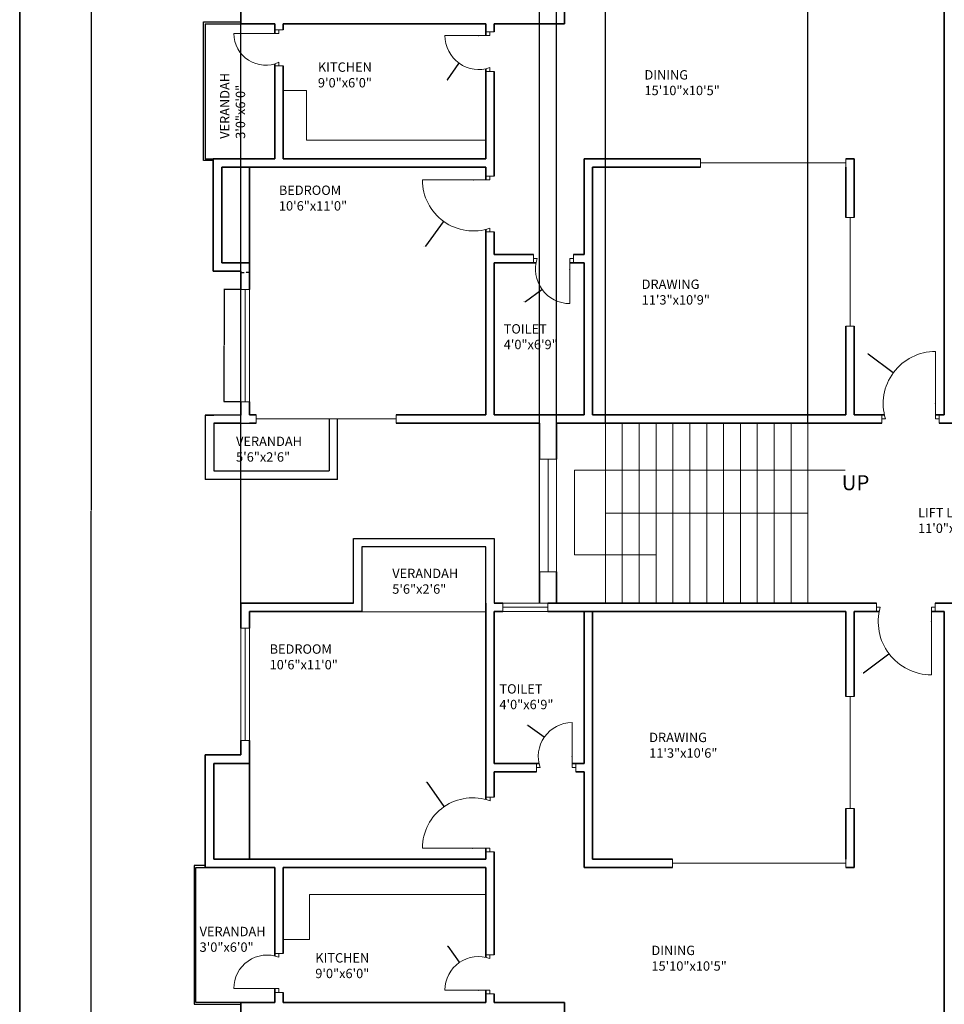
# Model space of a CAD drawing. Units: inches. Extents: x 2154 to 3131, y 1384 to 2688.
# Tile 2 of 5: x 2154 to 2647, y 1828 to 2353. Entities that reach past the tile are written whole.
import ezdxf

# ---------------------------------------------------------------- set-up
doc = ezdxf.new("R2010")
doc.units = ezdxf.units.IN
for name, color, linetype, lineweight in [('A-ANNO-DIMS', 2, 'Continuous', 18), ('A-ANNO-SYMB', 3, 'Continuous', 18), ('A-ANNO-TTLB', 7, 'Continuous', 35), ('A-AREA-IDEN', 7, 'Continuous', 18), ('A-DOOR', 31, 'Continuous', 18), ('A-FLOR-BALC', 130, 'Continuous', 25), ('A-FLOR-FIXT', 8, 'Continuous', 18), ('A-FLOR-STRS', 7, 'Continuous', 18), ('A-GLAZ', 130, 'Continuous', 18), ('A-WALL', 7, 'Continuous', 35)]:
    doc.layers.add(name, color=color, linetype=linetype, lineweight=lineweight)
doc.styles.get("Standard").update_dxf_attribs({"font": 'arial.ttf'})
doc.dimstyles.get("Standard").update_dxf_attribs({"dimtxt": 0.18, "dimasz": 0.18, "dimexe": 0.18, "dimexo": 0.0625, "dimgap": 0.09, "dimtad": 0, "dimtih": 1, "dimtoh": 1, "dimdec": 4, "dimzin": 0, "dimdsep": 46, "dimtxsty": 'Standard', "dimcen": 0.09, "dimadec": 0, "dimazin": 0, "dimtfac": 1, "dimtdec": 4, "dimtofl": 0, "dimtmove": 0, "dimatfit": 3, "dimfxl": 1, "dimtolj": 1, "dimtzin": 0, "dimarcsym": 0})

# ---------------------------------------------------------------- blocks, each defined once
blk = doc.blocks.new('DOOR-LEAF-24-JAMB-A')
for p, q in [((0, 2.25), (0, 26.25)), ((2, 2.25), (0, 2.25)), ((2, 4.5), (2, 0)), ((2, 0), (2, 2.25))]:
    blk.add_line(p, q)
blk = doc.blocks.new('DOOR-LEAF-36-JAMB-A')
for p, q in [((2, 2.25), (2, 38.25)), ((0, 4.5), (0, 0)), ((0, 0), (0, 2.25)), ((0, 2.25), (2, 2.25))]:
    blk.add_line(p, q)
blk = doc.blocks.new('DOOR-LEAF-24-JAMB-B')
for p, q in [((0, 2), (4.5, 2)), ((4.5, 2), (2.25, 2)), ((2.25, 2), (2.25, 0)), ((2.25, 0), (26.25, 0))]:
    blk.add_line(p, q)
blk = doc.blocks.new('WIN-24-FRAME-A')
for p, q in [((0, 4.5), (0, 0)), ((0, 4.5), (24, 4.5)), ((0, 0), (0, 2.25)), ((0, 2.25), (24, 2.25)), ((0, 0), (24, 0)), ((24, 2.25), (24, 4.5)), ((24, 4.5), (24, 0))]:
    blk.add_line(p, q)
blk = doc.blocks.new('WIN-60')
for p, q in [((2.25, 60), (0, 60)), ((0, 60), (4.5, 60)), ((0, 60), (0, 0)), ((2.25, 0), (2.25, 60)), ((4.5, 60), (4.5, 0)), ((0, 0), (4.5, 0)), ((4.5, 0), (2.25, 0))]:
    blk.add_line(p, q)
blk = doc.blocks.new('*D20')
at = {"layer": 'A-ANNO-DIMS', "color": 0, "lineweight": -2, "transparency": 16777216}
for p, q in [((2272.09, 2209.02), (2262.98, 2209.02)), ((2263.16, 2208.84), (2263.16, 2179.2)), ((2263.16, 2149.2), (2263.16, 2178.84)), ((2272.09, 2149.02), (2262.98, 2149.02))]:
    blk.add_line(p, q, dxfattribs=at)
at = {"layer": 'A-ANNO-DIMS', "color": 0, "transparency": 16777216}
for points in [[(2263.13, 2208.84), (2263.19, 2208.84), (2263.16, 2209.02)], [(2263.13, 2149.2), (2263.19, 2149.2), (2263.16, 2149.02)]]:
    blk.add_solid(points, dxfattribs=at)
at = {"layer": 'Defpoints', "color": 0, "transparency": 16777216}
for p in [(2272.16, 2209.02), (2263.16, 2149.02), (2272.16, 2149.02)]:
    blk.add_point(p, dxfattribs=at)
at = {"layer": 'A-ANNO-DIMS', "color": 0, "transparency": 16777216, "insert": (2263.16, 2179.02), "char_height": 0.18, "attachment_point": 5}
blk.add_mtext('\\A1;W3 60 TYP.', dxfattribs=at)
blk = doc.blocks.new('*D21')
at = {"layer": 'A-ANNO-DIMS', "color": 0, "lineweight": -2, "transparency": 16777216}
for p, q in [((2272.16, 2209.08), (2272.16, 2218.2)), ((2272.34, 2218.02), (2273.95, 2218.02)), ((2276.48, 2218.02), (2274.86, 2218.02)), ((2276.66, 2209.08), (2276.66, 2218.2))]:
    blk.add_line(p, q, dxfattribs=at)
at = {"layer": 'A-ANNO-DIMS', "color": 0, "transparency": 16777216}
for points in [[(2272.34, 2218.05), (2272.34, 2217.99), (2272.16, 2218.02)], [(2276.48, 2218.05), (2276.48, 2217.99), (2276.66, 2218.02)]]:
    blk.add_solid(points, dxfattribs=at)
at = {"layer": 'Defpoints', "color": 0, "transparency": 16777216}
for p in [(2272.16, 2218.02), (2272.16, 2209.02), (2276.66, 2209.02)]:
    blk.add_point(p, dxfattribs=at)
at = {"layer": 'A-ANNO-DIMS', "color": 0, "transparency": 16777216, "insert": (2274.41, 2218.02), "char_height": 0.18, "attachment_point": 5}
blk.add_mtext('\\A1;5 TYP.', dxfattribs=at)
blk = doc.blocks.new('*D23')
at = {"layer": 'A-ANNO-DIMS', "color": 0, "lineweight": -2, "transparency": 16777216}
for p, q in [((2504.09, 2580.68), (2192.08, 2580.68)), ((2192.26, 2580.5), (2192.26, 2091.11)), ((2192.26, 1601.36), (2192.26, 2090.74)), ((2504.09, 1601.18), (2192.08, 1601.18))]:
    blk.add_line(p, q, dxfattribs=at)
at = {"layer": 'A-ANNO-DIMS', "color": 0, "transparency": 16777216}
for points in [[(2192.23, 2580.5), (2192.29, 2580.5), (2192.26, 2580.68)], [(2192.23, 1601.36), (2192.29, 1601.36), (2192.26, 1601.18)]]:
    blk.add_solid(points, dxfattribs=at)
at = {"layer": 'Defpoints', "color": 0, "transparency": 16777216}
for p in [(2192.26, 2580.68), (2504.16, 2580.68), (2504.16, 1601.18)]:
    blk.add_point(p, dxfattribs=at)
at = {"layer": 'A-ANNO-DIMS', "color": 0, "transparency": 16777216, "insert": (2192.26, 2090.93), "char_height": 0.18, "attachment_point": 5}
blk.add_mtext('\\A1;979.5', dxfattribs=at)
blk = doc.blocks.new('*D26')
at = {"layer": 'A-ANNO-DIMS', "color": 0, "lineweight": -2, "transparency": 16777216}
for p, q in [((2272.16, 2041.74), (2272.16, 2635.76)), ((2272.34, 2635.58), (2351.32, 2635.58)), ((2431.22, 2635.58), (2352.24, 2635.58)), ((2431.4, 2041.74), (2431.4, 2635.76))]:
    blk.add_line(p, q, dxfattribs=at)
at = {"layer": 'A-ANNO-DIMS', "color": 0, "transparency": 16777216}
for points in [[(2272.34, 2635.61), (2272.34, 2635.55), (2272.16, 2635.58)], [(2431.22, 2635.61), (2431.22, 2635.55), (2431.4, 2635.58)]]:
    blk.add_solid(points, dxfattribs=at)
at = {"layer": 'Defpoints', "color": 0, "transparency": 16777216}
for p in [(2431.4, 2635.58), (2272.16, 2041.68), (2431.4, 2041.68)]:
    blk.add_point(p, dxfattribs=at)
at = {"layer": 'A-ANNO-DIMS', "color": 0, "transparency": 16777216, "insert": (2351.78, 2635.58), "char_height": 0.18, "attachment_point": 5}
blk.add_mtext('\\A1;159.25', dxfattribs=at)
blk = doc.blocks.new('*D28')
at = {"layer": 'A-ANNO-DIMS', "color": 0, "lineweight": -2, "transparency": 16777216}
for p, q in [((2466.46, 2137.74), (2466.46, 2635.76)), ((2466.64, 2635.58), (2520.18, 2635.58)), ((2574.28, 2635.58), (2520.74, 2635.58)), ((2574.46, 2137.74), (2574.46, 2635.76))]:
    blk.add_line(p, q, dxfattribs=at)
at = {"layer": 'A-ANNO-DIMS', "color": 0, "transparency": 16777216}
for points in [[(2466.64, 2635.61), (2466.64, 2635.55), (2466.46, 2635.58)], [(2574.28, 2635.61), (2574.28, 2635.55), (2574.46, 2635.58)]]:
    blk.add_solid(points, dxfattribs=at)
at = {"layer": 'Defpoints', "color": 0, "transparency": 16777216}
for p in [(2574.46, 2635.58), (2466.46, 2137.68), (2574.46, 2137.68)]:
    blk.add_point(p, dxfattribs=at)
at = {"layer": 'A-ANNO-DIMS', "color": 0, "transparency": 16777216, "insert": (2520.46, 2635.58), "char_height": 0.18, "attachment_point": 5}
blk.add_mtext('\\A1;108', dxfattribs=at)
blk = doc.blocks.new('*D29')
at = {"layer": 'A-ANNO-DIMS', "color": 0, "lineweight": -2, "transparency": 16777216}
for p, q in [((2440.4, 2137.74), (2440.4, 2635.76)), ((2440.58, 2635.58), (2453.04, 2635.58)), ((2466.28, 2635.58), (2453.83, 2635.58)), ((2466.46, 2137.74), (2466.46, 2635.76))]:
    blk.add_line(p, q, dxfattribs=at)
at = {"layer": 'A-ANNO-DIMS', "color": 0, "transparency": 16777216}
for points in [[(2440.58, 2635.61), (2440.58, 2635.55), (2440.4, 2635.58)], [(2466.28, 2635.61), (2466.28, 2635.55), (2466.46, 2635.58)]]:
    blk.add_solid(points, dxfattribs=at)
at = {"layer": 'Defpoints', "color": 0, "transparency": 16777216}
for p in [(2466.46, 2635.58), (2440.4, 2137.68), (2466.46, 2137.68)]:
    blk.add_point(p, dxfattribs=at)
at = {"layer": 'A-ANNO-DIMS', "color": 0, "transparency": 16777216, "insert": (2453.43, 2635.58), "char_height": 0.18, "attachment_point": 5}
blk.add_mtext('\\A1;26.06', dxfattribs=at)
blk = doc.blocks.new('*D44')
at = {"layer": 'A-ANNO-DIMS', "color": 0, "lineweight": -2, "transparency": 16777216}
for p, q in [((2396.02, 2267.4), (2396.2, 2267.4)), ((2396.11, 2267.31), (2396.11, 2267.49)), ((2370.78, 2231.99), (2380.18, 2245.12)), ((2370.6, 2231.99), (2370.78, 2231.99))]:
    blk.add_line(p, q, dxfattribs=at)
at = {"layer": 'A-ANNO-DIMS', "color": 0, "transparency": 16777216}
blk.add_solid([(2380.15, 2245.14), (2380.2, 2245.1), (2380.28, 2245.27)], dxfattribs=at)
at = {"layer": 'Defpoints', "color": 0, "transparency": 16777216}
for p in [(2396.11, 2267.4), (2380.28, 2245.27)]:
    blk.add_point(p, dxfattribs=at)
at = {"layer": 'A-ANNO-DIMS', "color": 0, "transparency": 16777216, "insert": (2370.05, 2231.99), "char_height": 0.18, "attachment_point": 5}
blk.add_mtext('\\A1;R27.207', dxfattribs=at)
blk = doc.blocks.new('*D45')
at = {"layer": 'A-ANNO-DIMS', "color": 0, "lineweight": -2, "transparency": 16777216}
for p, q in [((2640.17, 2031.74), (2640.35, 2031.74)), ((2640.26, 2031.65), (2640.26, 2031.83)), ((2604.14, 2004.4), (2617.54, 2014.54)), ((2603.96, 2004.4), (2604.14, 2004.4))]:
    blk.add_line(p, q, dxfattribs=at)
at = {"layer": 'A-ANNO-DIMS', "color": 0, "transparency": 16777216}
blk.add_solid([(2617.52, 2014.57), (2617.56, 2014.52), (2617.68, 2014.65)], dxfattribs=at)
at = {"layer": 'Defpoints', "color": 0, "transparency": 16777216}
for p in [(2640.26, 2031.74), (2617.68, 2014.65)]:
    blk.add_point(p, dxfattribs=at)
at = {"layer": 'A-ANNO-DIMS', "color": 0, "transparency": 16777216, "insert": (2603.5, 2004.4), "char_height": 0.18, "attachment_point": 5}
blk.add_mtext('\\A1;R28.31', dxfattribs=at)
blk = doc.blocks.new('*D46')
at = {"layer": 'A-ANNO-DIMS', "color": 0, "lineweight": -2, "transparency": 16777216}
for p, q in [((2606.44, 2174.61), (2606.62, 2174.61)), ((2606.62, 2174.61), (2619.92, 2164.75)), ((2642.38, 2148.03), (2642.56, 2148.03)), ((2642.47, 2147.94), (2642.47, 2148.12))]:
    blk.add_line(p, q, dxfattribs=at)
at = {"layer": 'A-ANNO-DIMS', "color": 0, "transparency": 16777216}
blk.add_solid([(2619.93, 2164.78), (2619.9, 2164.73), (2620.06, 2164.65)], dxfattribs=at)
at = {"layer": 'Defpoints', "color": 0, "transparency": 16777216}
for p in [(2620.06, 2164.65), (2642.47, 2148.03)]:
    blk.add_point(p, dxfattribs=at)
at = {"layer": 'A-ANNO-DIMS', "color": 0, "transparency": 16777216, "insert": (2605.89, 2174.61), "char_height": 0.18, "attachment_point": 5}
blk.add_mtext('\\A1;R27.893', dxfattribs=at)
blk = doc.blocks.new('*D50')
at = {"layer": 'A-ANNO-DIMS', "color": 0, "lineweight": -2, "transparency": 16777216}
for p, q in [((2371, 1946.2), (2371.18, 1946.2)), ((2371.18, 1946.2), (2380.28, 1933.15)), ((2395.62, 1911.01), (2395.8, 1911.01)), ((2395.71, 1910.92), (2395.71, 1911.1))]:
    blk.add_line(p, q, dxfattribs=at)
at = {"layer": 'A-ANNO-DIMS', "color": 0, "transparency": 16777216}
blk.add_solid([(2380.3, 1933.17), (2380.25, 1933.13), (2380.38, 1933)], dxfattribs=at)
at = {"layer": 'Defpoints', "color": 0, "transparency": 16777216}
for p in [(2380.38, 1933), (2395.71, 1911.01)]:
    blk.add_point(p, dxfattribs=at)
at = {"layer": 'A-ANNO-DIMS', "color": 0, "transparency": 16777216, "insert": (2370.45, 1946.2), "char_height": 0.18, "attachment_point": 5}
blk.add_mtext('\\A1;R26.807', dxfattribs=at)
blk = doc.blocks.new('*D61')
at = {"layer": 'A-ANNO-DIMS', "color": 0, "lineweight": -2, "transparency": 16777216}
for p, q in [((2447.41, 2219.74), (2447.59, 2219.74)), ((2447.5, 2219.65), (2447.5, 2219.83)), ((2423.78, 2202.54), (2432.53, 2208.88)), ((2423.6, 2202.54), (2423.78, 2202.54))]:
    blk.add_line(p, q, dxfattribs=at)
at = {"layer": 'A-ANNO-DIMS', "color": 0, "transparency": 16777216}
blk.add_solid([(2432.51, 2208.91), (2432.55, 2208.86), (2432.68, 2208.99)], dxfattribs=at)
at = {"layer": 'Defpoints', "color": 0, "transparency": 16777216}
for p in [(2447.5, 2219.74), (2432.68, 2208.99)]:
    blk.add_point(p, dxfattribs=at)
at = {"layer": 'A-ANNO-DIMS', "color": 0, "transparency": 16777216, "insert": (2423.14, 2202.54), "char_height": 0.18, "attachment_point": 5}
blk.add_mtext('\\A1;R18.31', dxfattribs=at)
blk = doc.blocks.new('*D62')
at = {"layer": 'A-ANNO-DIMS', "color": 0, "lineweight": -2, "transparency": 16777216}
for p, q in [((2398.89, 2344.39), (2399.07, 2344.39)), ((2398.98, 2344.3), (2398.98, 2344.48)), ((2382.2, 2320.82), (2388.39, 2329.51)), ((2382.02, 2320.82), (2382.2, 2320.82))]:
    blk.add_line(p, q, dxfattribs=at)
at = {"layer": 'A-ANNO-DIMS', "color": 0, "transparency": 16777216}
blk.add_solid([(2388.37, 2329.53), (2388.42, 2329.49), (2388.49, 2329.66)], dxfattribs=at)
at = {"layer": 'Defpoints', "color": 0, "transparency": 16777216}
for p in [(2398.98, 2344.39), (2388.49, 2329.66)]:
    blk.add_point(p, dxfattribs=at)
at = {"layer": 'A-ANNO-DIMS', "color": 0, "transparency": 16777216, "insert": (2381.47, 2320.82), "char_height": 0.18, "attachment_point": 5}
blk.add_mtext('\\A1;R18.082', dxfattribs=at)
blk = doc.blocks.new('*D63')
at = {"layer": 'A-ANNO-DIMS', "color": 0, "lineweight": -2, "transparency": 16777216}
for p, q in [((2424.99, 1976.53), (2425.17, 1976.53)), ((2425.17, 1976.53), (2433.84, 1970.42)), ((2448.58, 1959.96), (2448.76, 1959.96)), ((2448.67, 1959.87), (2448.67, 1960.05))]:
    blk.add_line(p, q, dxfattribs=at)
at = {"layer": 'A-ANNO-DIMS', "color": 0, "transparency": 16777216}
blk.add_solid([(2433.85, 1970.44), (2433.82, 1970.39), (2433.98, 1970.31)], dxfattribs=at)
at = {"layer": 'Defpoints', "color": 0, "transparency": 16777216}
for p in [(2433.98, 1970.31), (2448.67, 1959.96)]:
    blk.add_point(p, dxfattribs=at)
at = {"layer": 'A-ANNO-DIMS', "color": 0, "transparency": 16777216, "insert": (2424.44, 1976.53), "char_height": 0.18, "attachment_point": 5}
blk.add_mtext('\\A1;R17.968', dxfattribs=at)
blk = doc.blocks.new('*D64')
at = {"layer": 'A-ANNO-DIMS', "color": 0, "lineweight": -2, "transparency": 16777216}
for p, q in [((2382.23, 1858.7), (2382.41, 1858.7)), ((2382.41, 1858.7), (2388.43, 1850.07)), ((2398.65, 1835.29), (2398.83, 1835.29)), ((2398.74, 1835.2), (2398.74, 1835.38))]:
    blk.add_line(p, q, dxfattribs=at)
at = {"layer": 'A-ANNO-DIMS', "color": 0, "transparency": 16777216}
blk.add_solid([(2388.45, 1850.08), (2388.41, 1850.05), (2388.53, 1849.92)], dxfattribs=at)
at = {"layer": 'Defpoints', "color": 0, "transparency": 16777216}
for p in [(2388.53, 1849.92), (2398.74, 1835.29)]:
    blk.add_point(p, dxfattribs=at)
at = {"layer": 'A-ANNO-DIMS', "color": 0, "transparency": 16777216, "insert": (2381.68, 1858.7), "char_height": 0.18, "attachment_point": 5}
blk.add_mtext('\\A1;R17.836', dxfattribs=at)

msp = doc.modelspace()

# ---------------------------------------------------------------- linework, layer by layer
at = {"layer": 'A-ANNO-SYMB'}
for p, q in [((2594.3022, 2112.5937), (2450.0628, 2112.5937)), ((2450.0628, 2112.5937), (2450.0628, 2067.4511)), ((2450.0628, 2067.4511), (2493.4638, 2067.4511))]:
    msp.add_line(p, q, dxfattribs=at)
at = {"layer": 'A-ANNO-TTLB'}
msp.add_lwpolyline([(2154.1953, 2688.4009), (3131.1627, 2688.4009), (3131.1627, 1383.7377), (2154.1953, 1383.7377)], close=True, dxfattribs=at)
at = {"layer": 'A-DOOR'}
for p, q in [((2290.1496, 2328.1708), (2294.6496, 2328.1708)), ((2292.3996, 2328.1708), (2292.3996, 2330.1708)), ((2294.6496, 2328.1708), (2292.3996, 2328.1708)), ((2294.6496, 2328.1708), (2294.6496, 2328.1708)), ((2404.8996, 2325.3014), (2404.8996, 2327.3014)), ((2402.6496, 2325.3014), (2407.1496, 2325.3014)), ((2407.1496, 2325.3014), (2404.8996, 2325.3014)), ((2402.6496, 2239.6489), (2407.1496, 2239.6489)), ((2404.8996, 2239.6489), (2404.8996, 2241.6489)), ((2407.1496, 2239.6489), (2404.8996, 2239.6489)), ((2428.0981, 2223.1767), (2428.0981, 2227.6767)), ((2428.0981, 2227.6767), (2428.0981, 2225.4267)), ((2428.0981, 2225.4267), (2428.0981, 2225.4267)), ((2428.0981, 2225.4267), (2430.0981, 2225.4267)), ((2613.778, 2142.1767), (2613.778, 2137.6767)), ((2613.778, 2137.6767), (2613.778, 2139.9267)), ((2613.778, 2139.9267), (2615.778, 2139.9267)), ((2611.0121, 2037.1767), (2611.0121, 2041.6767)), ((2611.0121, 2041.6767), (2611.0121, 2039.4267)), ((2611.0121, 2039.4267), (2613.0121, 2039.4267)), ((2429.743, 1956.1767), (2429.743, 1951.6767)), ((2429.743, 1951.6767), (2429.743, 1953.9267)), ((2429.743, 1953.9267), (2431.743, 1953.9267)), ((2402.656, 1938.1684), (2405.7918, 1938.1684)), ((2407.156, 1938.1684), (2404.981, 1938.1684)), ((2404.981, 1938.1684), (2404.981, 1936.1684)), ((2405.7918, 1938.1684), (2407.156, 1938.1684)), ((2290.1496, 1854.7927), (2294.6496, 1854.7927)), ((2294.6496, 1854.7927), (2292.3996, 1854.7927)), ((2292.3996, 1854.7927), (2292.3996, 1852.7927)), ((2402.6496, 1854.0259), (2407.1496, 1854.0259)), ((2407.1496, 1854.0259), (2404.8996, 1854.0259)), ((2404.8996, 1854.0259), (2404.8996, 1852.0259))]:
    msp.add_line(p, q, dxfattribs=at)
for centre, radius, start, end in [((2285.2686, 2345.4584), 16.869, 180, 295.006893), ((2398.9816, 2344.3876), 18.082, 180, 289.10408), ((2396.1067, 2267.3958), 27.207, 180, 288.855792), ((2447.4998, 2219.7354), 18.3087, 161.889545, 270), ((2642.4666, 2148.0339), 27.8928, 90, 196.897235), ((2640.2555, 2031.7351), 28.3084, 164.234141, 270), ((2448.6681, 1959.9588), 17.9679, 90, 199.616055), ((2395.7127, 1911.0149), 26.8067, 69.772734, 180), ((2286.1204, 1836.2206), 17.7218, 69.248023, 180.607644), ((2398.7355, 1835.2891), 17.8359, 69.781348, 180)]:
    msp.add_arc(centre, radius, start, end, dxfattribs=at)
at = {"layer": 'A-FLOR-BALC'}
for p, q in [((2252.1496, 2350.6767), (2252.1496, 2351.6767)), ((2252.1496, 2351.6767), (2272.156, 2351.6767)), ((2252.1496, 2277.6767), (2252.1496, 2350.6767)), ((2253.1496, 2350.6767), (2253.1496, 2278.6767)), ((2253.1496, 2350.6767), (2272.156, 2350.6767)), ((2253.1496, 2277.6767), (2252.1496, 2277.6767)), ((2253.1496, 2278.6767), (2257.3771, 2278.6767)), ((2257.3771, 2277.6767), (2253.1496, 2277.6767)), ((2257.3771, 2278.6767), (2257.3771, 2278.6767)), ((2257.3771, 2278.6767), (2257.3771, 2277.6767)), ((2272.156, 2141.9626), (2253.1496, 2141.9626)), ((2253.1496, 2141.9626), (2253.1496, 2137.6767)), ((2253.1496, 2141.9626), (2257.6496, 2141.9626)), ((2253.1496, 2141.9626), (2253.1496, 2137.6767)), ((2253.1496, 2137.6767), (2253.1496, 2107.6767)), ((2272.156, 2137.6767), (2257.6496, 2137.6767)), ((2257.6496, 2137.6767), (2280.2234, 2137.6767)), ((2257.6496, 2137.6767), (2257.6496, 2112.1767)), ((2319.1496, 2139.9267), (2319.1496, 2112.1767)), ((2323.6496, 2107.6767), (2323.6496, 2139.9267)), ((2257.6496, 2112.1767), (2319.1496, 2112.1767)), ((2323.6496, 2107.6767), (2253.1496, 2107.6767)), ((2332.156, 2071.6767), (2332.156, 2076.1767)), ((2332.156, 2076.1767), (2402.656, 2076.1767)), ((2402.656, 2076.1767), (2407.156, 2076.1767)), ((2407.156, 2076.1767), (2407.156, 2041.6767)), ((2332.156, 2041.6767), (2332.156, 2071.6767)), ((2402.656, 2071.6767), (2336.656, 2071.6767)), ((2336.656, 2071.6767), (2336.656, 2037.1767)), ((2402.656, 2041.6767), (2402.656, 2071.6767)), ((2402.656, 2041.6767), (2402.656, 2037.0296)), ((2336.656, 2037.1767), (2402.656, 2037.0296)), ((2248.156, 1901.6767), (2247.156, 1901.6767)), ((2247.156, 1901.6767), (2247.156, 1827.6767)), ((2253.1496, 1901.6767), (2248.156, 1901.6767)), ((2253.1496, 1900.6767), (2253.1496, 1901.6767)), ((2248.156, 1828.6767), (2248.156, 1900.6767)), ((2248.156, 1900.6767), (2252.7937, 1900.6767)), ((2252.7937, 1900.6767), (2253.1496, 1900.6767)), ((2247.156, 1827.6767), (2272.156, 1827.6767)), ((2272.156, 1828.6767), (2248.156, 1828.6767))]:
    msp.add_line(p, q, dxfattribs=at)
at = {"layer": 'A-FLOR-FIXT'}
for p, q in [((2294.6496, 2315.0562), (2307.1795, 2315.0562)), ((2307.1795, 2315.0562), (2307.1795, 2288.5564)), ((2307.1795, 2288.5564), (2402.6496, 2288.5564)), ((2308.6982, 1862.1752), (2308.6982, 1886.2747)), ((2308.6982, 1886.2747), (2402.6496, 1886.2747)), ((2294.6496, 1862.1752), (2308.6982, 1862.1752))]:
    msp.add_line(p, q, dxfattribs=at)
at = {"layer": 'A-FLOR-STRS'}
for p, q in [((2466.4638, 2137.6767), (2466.4638, 2041.6767)), ((2475.4638, 2137.6767), (2475.4638, 2041.6767)), ((2484.4638, 2137.6767), (2484.4638, 2041.6767)), ((2493.4638, 2137.6767), (2493.4638, 2041.6767)), ((2502.4638, 2137.6767), (2502.4638, 2041.6767)), ((2511.4638, 2137.6767), (2511.4638, 2041.6767)), ((2520.4638, 2137.6767), (2520.4638, 2041.6767)), ((2529.4638, 2137.6767), (2529.4638, 2041.6767)), ((2538.4638, 2137.6767), (2538.4638, 2041.6767)), ((2547.4638, 2137.6767), (2547.4638, 2041.6767)), ((2556.4638, 2137.6767), (2556.4638, 2041.6767)), ((2565.4638, 2137.6767), (2565.4638, 2041.6767)), ((2574.4638, 2137.6767), (2574.4638, 2041.6767)), ((2466.4638, 2089.6767), (2574.4638, 2089.6767))]:
    msp.add_line(p, q, dxfattribs=at)
at = {"layer": 'A-GLAZ'}
for p, q in [((2517.2413, 2278.6767), (2517.2413, 2274.1767)), ((2594.6496, 2276.4267), (2517.2413, 2276.4267)), ((2594.6496, 2274.1767), (2594.6496, 2278.6767)), ((2594.6496, 2278.6767), (2594.6496, 2276.4267)), ((2596.8996, 2247.4008), (2594.6496, 2247.4008)), ((2594.6496, 2247.4008), (2599.1496, 2247.4008)), ((2596.8996, 2189.4501), (2596.8996, 2247.4008)), ((2594.6496, 2189.4501), (2599.1496, 2189.4501)), ((2599.1496, 2189.4501), (2596.8996, 2189.4501)), ((2280.2234, 2139.9267), (2280.2234, 2142.1767)), ((2280.2234, 2142.1767), (2280.2234, 2137.6767)), ((2316.5987, 2139.9267), (2280.2234, 2139.9267)), ((2354.9376, 2139.9267), (2316.5987, 2139.9267)), ((2354.9376, 2137.6767), (2354.9376, 2142.1767)), ((2354.9376, 2142.1767), (2354.9376, 2139.9267)), ((2431.4046, 2118.369), (2440.4046, 2118.369)), ((2431.4046, 2118.369), (2431.4046, 2058.369)), ((2440.4046, 2118.369), (2435.9046, 2118.369)), ((2435.9046, 2118.369), (2435.9046, 2082.369)), ((2440.4046, 2118.369), (2440.4046, 2058.369)), ((2435.9046, 2082.369), (2435.9046, 2058.369)), ((2435.9046, 2058.369), (2431.4046, 2058.369)), ((2431.4046, 2058.369), (2440.4046, 2058.369)), ((2411.8284, 2039.4267), (2411.8284, 2039.4267)), ((2594.656, 1991.7924), (2599.156, 1991.7924)), ((2599.156, 1991.7924), (2596.906, 1991.7924)), ((2596.906, 1991.7924), (2596.906, 1932.0522)), ((2599.156, 1932.0522), (2594.656, 1932.0522)), ((2596.906, 1932.0522), (2599.156, 1932.0522)), ((2502.2218, 1902.9267), (2502.2218, 1905.1767)), ((2502.2218, 1905.1767), (2502.2218, 1900.6767)), ((2594.656, 1902.9267), (2502.2218, 1902.9267)), ((2594.656, 1905.1767), (2594.656, 1900.6767)), ((2594.656, 1900.6767), (2594.656, 1902.9267))]:
    msp.add_line(p, q, dxfattribs=at)
at = {"layer": 'A-WALL'}
for p, q in [((2647.156, 2400.1767), (2647.156, 2142.1767)), ((2272.156, 2364.3207), (2272.156, 2350.6767)), ((2444.656, 2358.253), (2444.656, 2350.6767)), ((2272.156, 2350.6767), (2290.1496, 2350.6767)), ((2290.1496, 2345.4584), (2290.1496, 2350.6767)), ((2294.6496, 2350.6767), (2294.6496, 2347.4584)), ((2294.6496, 2350.6767), (2402.6496, 2350.6767)), ((2402.6496, 2350.6767), (2402.6496, 2344.3876)), ((2407.1496, 2350.6767), (2407.1496, 2346.3876)), ((2407.1496, 2350.6767), (2444.656, 2350.6767)), ((2290.1496, 2278.6767), (2290.1496, 2329.311)), ((2294.6496, 2328.1708), (2294.6496, 2278.6767)), ((2402.6496, 2326.6815), (2402.6496, 2278.6767)), ((2407.1496, 2325.3014), (2407.1496, 2274.1767)), ((2276.656, 2278.6767), (2257.3771, 2278.6767)), ((2257.3771, 2278.6767), (2257.3771, 2242.6767)), ((2276.656, 2274.1767), (2261.8771, 2274.1767)), ((2261.8771, 2274.1767), (2261.8771, 2223.1767)), ((2276.656, 2278.6767), (2290.1496, 2278.6767)), ((2276.656, 2274.1767), (2402.6496, 2274.1767)), ((2276.656, 2223.1767), (2276.656, 2274.1767)), ((2294.6496, 2278.6767), (2402.6496, 2278.6767)), ((2402.6496, 2267.3958), (2402.6496, 2274.1767)), ((2407.1496, 2274.1767), (2407.1496, 2269.3958)), ((2455.1496, 2278.6767), (2517.2413, 2278.6767)), ((2455.1496, 2278.6767), (2455.1496, 2227.6767)), ((2517.2413, 2278.6767), (2455.1496, 2278.6767)), ((2459.6496, 2274.1767), (2517.2413, 2274.1767)), ((2459.6496, 2274.1767), (2459.6496, 2142.1767)), ((2599.1496, 2278.6767), (2594.6496, 2278.6767)), ((2594.6496, 2278.6767), (2599.1496, 2278.6767)), ((2594.6496, 2274.1767), (2594.6496, 2247.4008)), ((2599.1496, 2278.6767), (2599.1496, 2247.4008)), ((2257.3771, 2242.6767), (2257.3771, 2218.6767)), ((2402.6496, 2142.1767), (2402.6496, 2240.9873)), ((2407.1496, 2239.6489), (2407.1496, 2227.6767)), ((2407.1496, 2227.6767), (2428.0981, 2227.6767)), ((2449.4998, 2227.6767), (2455.1496, 2227.6767)), ((2261.8771, 2223.1767), (2276.656, 2223.1767)), ((2276.656, 2223.1767), (2276.656, 2218.6767)), ((2407.1496, 2223.1767), (2429.5174, 2223.1767)), ((2407.1496, 2223.1767), (2407.1496, 2142.1767)), ((2447.4998, 2223.1767), (2455.1496, 2223.1767)), ((2455.1496, 2223.1767), (2455.1496, 2142.1767)), ((2257.3771, 2218.6767), (2272.156, 2218.6767)), ((2272.156, 2218.6767), (2272.156, 2209.0196)), ((2276.656, 2218.6767), (2276.656, 2209.0196)), ((2594.6496, 2189.4501), (2594.6496, 2142.1767)), ((2599.1496, 2189.4501), (2599.1496, 2142.1767)), ((2272.156, 2149.0196), (2272.156, 2141.9626)), ((2276.656, 2149.0196), (2276.656, 2142.1767)), ((2276.656, 2142.1767), (2280.2234, 2142.1767)), ((2276.656, 2137.6767), (2280.2234, 2137.6767)), ((2354.9376, 2142.1767), (2402.6496, 2142.1767)), ((2354.9376, 2137.6767), (2431.4046, 2137.6767)), ((2407.1496, 2137.6767), (2402.6496, 2137.6767)), ((2407.1496, 2142.1767), (2455.1496, 2142.1767)), ((2431.4046, 2137.6767), (2431.4046, 2118.369)), ((2440.4046, 2137.6767), (2440.4046, 2118.369)), ((2440.4046, 2137.6767), (2613.778, 2137.6767)), ((2459.6496, 2142.1767), (2594.6496, 2142.1767)), ((2599.1496, 2142.1767), (2615.1958, 2142.1767)), ((2642.4666, 2142.1767), (2647.156, 2142.1767)), ((2644.4666, 2137.6767), (2655.7665, 2137.6767)), ((2431.4046, 2058.369), (2431.4046, 2041.6767)), ((2440.4046, 2058.369), (2440.4046, 2041.6767)), ((2272.156, 2041.6767), (2272.156, 2028.3598)), ((2272.156, 2041.6767), (2332.156, 2041.6767)), ((2402.656, 2041.6767), (2402.656, 1936.9068)), ((2407.156, 2041.6767), (2411.8284, 2041.6767)), ((2435.8284, 2041.6767), (2440.4046, 2041.6767)), ((2440.4046, 2041.6767), (2611.0121, 2041.6767)), ((2574.4638, 2041.6767), (2611.0121, 2041.6767)), ((2642.2555, 2041.6767), (2647.156, 2041.6767)), ((2642.2555, 2041.6767), (2654.6623, 2041.6767)), ((2276.656, 2037.1767), (2336.656, 2037.1767)), ((2276.656, 2037.1767), (2336.656, 2037.1767)), ((2276.656, 2037.1767), (2276.656, 2028.3598)), ((2407.156, 2037.1767), (2411.8284, 2037.1767)), ((2407.156, 2037.1767), (2411.8284, 2037.1767)), ((2407.156, 1956.1767), (2407.156, 2037.1767)), ((2435.8284, 2037.1767), (2455.156, 2037.1767)), ((2435.8284, 2037.1767), (2594.656, 2037.1767)), ((2455.156, 2037.1767), (2455.156, 1956.1767)), ((2459.656, 1905.1767), (2459.656, 2037.1767)), ((2459.656, 2037.1767), (2594.656, 2037.1767)), ((2594.656, 2037.1767), (2594.656, 1991.7924)), ((2599.156, 2037.1767), (2612.475, 2037.1767)), ((2599.156, 1991.7924), (2599.156, 2037.1767)), ((2640.2555, 2037.1767), (2647.156, 2037.1767)), ((2647.156, 2037.1767), (2647.156, 1782.1799)), ((2272.156, 1968.3598), (2272.156, 1960.6767)), ((2276.656, 1968.3598), (2276.656, 1956.1767)), ((2253.1496, 1900.6767), (2253.1496, 1960.6767)), ((2253.1496, 1960.6767), (2272.156, 1960.6767)), ((2276.656, 1960.6767), (2276.656, 1956.1767)), ((2276.656, 1956.1767), (2257.6496, 1956.1767)), ((2257.6496, 1956.1767), (2257.6496, 1905.1767)), ((2276.656, 1956.1767), (2276.656, 1905.1767)), ((2407.156, 1956.1767), (2431.1028, 1956.1767)), ((2448.6681, 1956.1767), (2455.156, 1956.1767)), ((2407.156, 1951.6767), (2429.743, 1951.6767)), ((2407.156, 1938.1684), (2407.156, 1951.6767)), ((2450.6681, 1951.6767), (2455.156, 1951.6767)), ((2455.156, 1951.6767), (2455.156, 1900.6767)), ((2594.656, 1932.0522), (2594.656, 1905.1767)), ((2599.156, 1900.6767), (2599.156, 1932.0522)), ((2402.656, 1911.0149), (2402.656, 1905.1767)), ((2407.156, 1900.6767), (2407.156, 1909.0149)), ((2257.6496, 1905.1767), (2272.156, 1905.1767)), ((2272.156, 1905.1767), (2402.656, 1905.1767)), ((2459.656, 1905.1767), (2502.2218, 1905.1767)), ((2272.156, 1900.6767), (2253.1496, 1900.6767)), ((2272.156, 1900.6767), (2290.1496, 1900.6767)), ((2290.1496, 1900.6767), (2290.1496, 1853.4783)), ((2294.6496, 1900.6767), (2402.6496, 1900.6767)), ((2294.6496, 1854.7927), (2294.6496, 1900.6767)), ((2294.6496, 1900.6767), (2402.6496, 1900.6767)), ((2402.6496, 1900.6767), (2402.6496, 1852.6902)), ((2407.1496, 1854.0259), (2407.1496, 1900.6767)), ((2407.1496, 1900.6767), (2407.156, 1900.6767)), ((2455.156, 1900.6767), (2502.2218, 1900.6767)), ((2594.656, 1900.6767), (2599.156, 1900.6767)), ((2290.1496, 1836.0327), (2290.1496, 1828.6767)), ((2294.6496, 1828.6767), (2294.6496, 1834.0327)), ((2402.6496, 1835.2891), (2402.6496, 1828.6767)), ((2407.1496, 1828.6767), (2407.1496, 1833.2891)), ((2272.156, 1828.6767), (2290.1496, 1828.6767)), ((2272.156, 1828.6767), (2272.156, 1746.1767)), ((2294.6496, 1828.6767), (2402.6496, 1828.6767)), ((2407.1496, 1828.6767), (2407.156, 1828.6767)), ((2407.156, 1828.6767), (2440.156, 1828.6767)), ((2440.156, 1828.6767), (2440.156, 1828.6767)), ((2440.156, 1828.6767), (2444.656, 1828.6767)), ((2444.656, 1828.6767), (2444.656, 1816.6226))]:
    msp.add_line(p, q, dxfattribs=at)

# ---------------------------------------------------------------- block references
at = {"layer": 'A-DOOR'}
for name, p, rotation in [('DOOR-LEAF-24-JAMB-A', (2294.6496, 2345.4584), 90.00000000000138), ('DOOR-LEAF-36-JAMB-A', (2642.2555, 2041.6767), 180), ('DOOR-LEAF-36-JAMB-A', (2407.156, 1909.0149), 90.00000000000036)]:
    msp.add_blockref(name, p, dxfattribs=dict(at, rotation=rotation))
at = {"layer": 'A-DOOR', "extrusion": (0, 0, -1), "zscale": -1}
for name, p in [('DOOR-LEAF-24-JAMB-B', (-2407.1496, 2344.3876)), ('DOOR-LEAF-36-JAMB-A', (-2644.4666, 2137.6767))]:
    msp.add_blockref(name, p, dxfattribs=at)
for name, p, rotation in [('DOOR-LEAF-36-JAMB-A', (-2407.1496, 2269.3958), 270.0000000000008), ('DOOR-LEAF-24-JAMB-A', (-2447.4998, 2227.6767), 180), ('DOOR-LEAF-24-JAMB-A', (-2294.6496, 1836.0327), 269.9999999999995), ('DOOR-LEAF-24-JAMB-A', (-2407.1496, 1835.2891), 270.0000000000002)]:
    msp.add_blockref(name, p, dxfattribs=dict(at, rotation=rotation))
at = {"layer": 'A-DOOR'}
msp.add_blockref('DOOR-LEAF-24-JAMB-A', (2448.6681, 1951.6767), dxfattribs=at)
at = {"layer": 'A-GLAZ', "rotation": 180}
for p in [(2276.656, 2209.0196), (2276.656, 2028.3598)]:
    msp.add_blockref('WIN-60', p, dxfattribs=at)
at = {"layer": 'A-GLAZ'}
msp.add_blockref('WIN-24-FRAME-A', (2411.8284, 2037.1767), dxfattribs=at)

# ---------------------------------------------------------------- texts
at = {"layer": 'A-ANNO-SYMB', "insert": (2592.4494, 2109.9038), "char_height": 8, "attachment_point": 1}
msp.add_mtext_dynamic_manual_height_columns('UP', width=35.445619, gutter_width=12.5, heights=[0], dxfattribs=at)
at = {"layer": 'A-AREA-IDEN', "char_height": 5, "attachment_point": 1}
for s, width, insert in [('KITCHEN\\P9\'0"x6\'0"', 175.939602, (2313.1876, 2330.0731)), ('DINING\\P15\'10"x10\'5"', 306.507323, (2487.3017, 2325.947)), ('BEDROOM\\P10\'6"x11\'0"', 184.441767, (2292.3989, 2264.3949)), ('DRAWING\\P11\'3"x10\'9"', 189.614125, (2485.8192, 2214.2478)), ('TOILET\\P4\'0"x6\'9"', 129.81334, (2412.2546, 2190.4518)), ('VERANDAH\\P5\'6"x2\'6"', 146.107868, (2269.5548, 2130.4582)), ('LIFT LOBBY\\P11\'0"x8\'0"', 149.609015, (2633.1561, 2092.4357)), ('VERANDAH\\P5\'6"x2\'6"', 146.107868, (2352.8309, 2060.0111)), ('BEDROOM\\P10\'6"x11\'0"', 177.832471, (2287.4453, 2019.6694)), ('TOILET\\P4\'0"x6\'9"', 160.716184, (2409.9695, 1998.4136)), ('DRAWING\\P11\'3"x10\'6"', 221.188944, (2489.8227, 1972.5457)), ('VERANDAH\\P3\'0"x6\'0"', 113.896015, (2250.1166, 1869.0036)), ('KITCHEN\\P9\'0"x6\'0"', 183.320961, (2311.7909, 1854.9619)), ('DINING\\P15\'10"x10\'5"', 244.835501, (2491.0172, 1858.9377))]:
    msp.add_mtext_dynamic_manual_height_columns(s, width=width, gutter_width=12.5, heights=[0], dxfattribs=dict(at, insert=insert))
at = {"layer": 'A-AREA-IDEN', "insert": (2261.0472, 2289.3188), "char_height": 5, "attachment_point": 1, "rotation": 90}
msp.add_mtext_dynamic_manual_height_columns('VERANDAH\\P3\'0"x6\'0"', width=116.935568, gutter_width=12.5, heights=[0], dxfattribs=at)

# ---------------------------------------------------------------- dimensions: what is measured, and where the dimension line sits
at = {"layer": 'A-ANNO-DIMS'}
for base, p1, p2, override, picture, middle in [((2431.4046, 2635.5767), (2272.156, 2041.6767), (2431.4046, 2041.6767), {"dimdec": 2, "dimlfac": 1, "dimrnd": 0, "dimzin": 0, "dimdsep": 46, "dimlunit": 2}, '*D26', (2351.7803, 2635.5767)), ((2466.4638, 2635.5767), (2440.4046, 2137.6767), (2466.4638, 2137.6767), {"dimdec": 2, "dimlfac": 1, "dimrnd": 0, "dimzin": 0, "dimdsep": 46, "dimlunit": 2}, '*D29', (2453.4342, 2635.5767)), ((2574.4638, 2635.5767), (2466.4638, 2137.6767), (2574.4638, 2137.6767), {"dimdec": 0, "dimlfac": 1, "dimrnd": 0, "dimzin": 0, "dimdsep": 46, "dimlunit": 2}, '*D28', (2520.4638, 2635.5767))]:
    dim = msp.add_linear_dim(base=base, p1=p1, p2=p2, dimstyle='Standard', override=override, dxfattribs=at)
    dim.commit()
    dim.dimension.update_dxf_attribs({"geometry": picture, "text_midpoint": middle})
dim = msp.add_linear_dim(base=(2192.256, 2580.6767), p1=(2504.156, 1601.1767), p2=(2504.156, 2580.6767), angle=90, dimstyle='Standard', override={"dimdec": 1, "dimlfac": 1, "dimrnd": 0, "dimzin": 0, "dimdsep": 46, "dimlunit": 2}, dxfattribs=at)
dim.commit()
dim.dimension.update_dxf_attribs({"geometry": '*D23', "text_midpoint": (2192.256, 2090.9267)})
for center, mpoint, override, picture, middle in [((2398.9816, 2344.3876), (2388.495, 2329.657), {"dimdec": 3, "dimlfac": 1, "dimrnd": 0, "dimzin": 0, "dimdsep": 46, "dimlunit": 2}, '*D62', (2381.4742, 2320.8186)), ((2396.1067, 2267.3958), (2380.2799, 2245.2658), {"dimdec": 3, "dimlfac": 1, "dimrnd": 0, "dimzin": 0, "dimdsep": 46, "dimlunit": 2}, '*D44', (2370.0541, 2231.9879)), ((2447.4998, 2219.7354), (2432.6773, 2208.9882), {"dimdec": 2, "dimlfac": 1, "dimrnd": 0, "dimzin": 0, "dimdsep": 46, "dimlunit": 2}, '*D61', (2423.1413, 2202.5399)), ((2642.4666, 2148.0339), (2620.0597, 2164.6452), {"dimdec": 3, "dimlfac": 1, "dimrnd": 0, "dimzin": 0, "dimdsep": 46, "dimlunit": 2}, '*D46', (2605.8857, 2174.612)), ((2640.2555, 2031.7351), (2617.6819, 2014.6529), {"dimdec": 2, "dimlfac": 1, "dimrnd": 0, "dimzin": 0, "dimdsep": 46, "dimlunit": 2}, '*D45', (2603.4953, 2004.4037)), ((2448.6681, 1959.9588), (2433.9842, 1970.3139), {"dimdec": 3, "dimlfac": 1, "dimrnd": 0, "dimzin": 0, "dimdsep": 46, "dimlunit": 2}, '*D63', (2424.4439, 1976.5269)), ((2395.7127, 1911.0149), (2380.3808, 1933.0043), {"dimdec": 3, "dimlfac": 1, "dimrnd": 0, "dimzin": 0, "dimdsep": 46, "dimlunit": 2}, '*D50', (2370.4519, 1946.1979)), ((2398.7355, 1835.2891), (2388.5331, 1849.9188), {"dimdec": 3, "dimlfac": 1, "dimrnd": 0, "dimzin": 0, "dimdsep": 46, "dimlunit": 2}, '*D64', (2381.682, 1858.6967))]:
    dim = msp.add_radius_dim(center=center, mpoint=mpoint, dimstyle='Standard', override=override, dxfattribs=at)
    dim.commit()
    dim.dimension.update_dxf_attribs({"geometry": picture, "text_midpoint": middle, "dimtype": 164})
for base, p1, p2, angle, text, picture, middle in [((2272.1560159305, 2218.0195973656), (2276.6560159305, 2209.0195973656), (2272.1560159305, 2209.0195973656), 180, '<> TYP.', '*D21', (2274.4060159305, 2218.0195973656)), ((2263.156, 2149.0196), (2272.156, 2209.0196), (2272.156, 2149.0196), 270, 'W3 <> TYP.', '*D20', (2263.156, 2179.0196))]:
    dim = msp.add_linear_dim(base=base, p1=p1, p2=p2, angle=angle, text=text, dimstyle='Standard', override={"dimdec": 0, "dimlfac": 1, "dimrnd": 0, "dimzin": 0, "dimdsep": 46, "dimlunit": 2}, dxfattribs=at)
    dim.commit()
    dim.dimension.update_dxf_attribs({"geometry": picture, "text_midpoint": middle})

doc.saveas('drawing.dxf')
